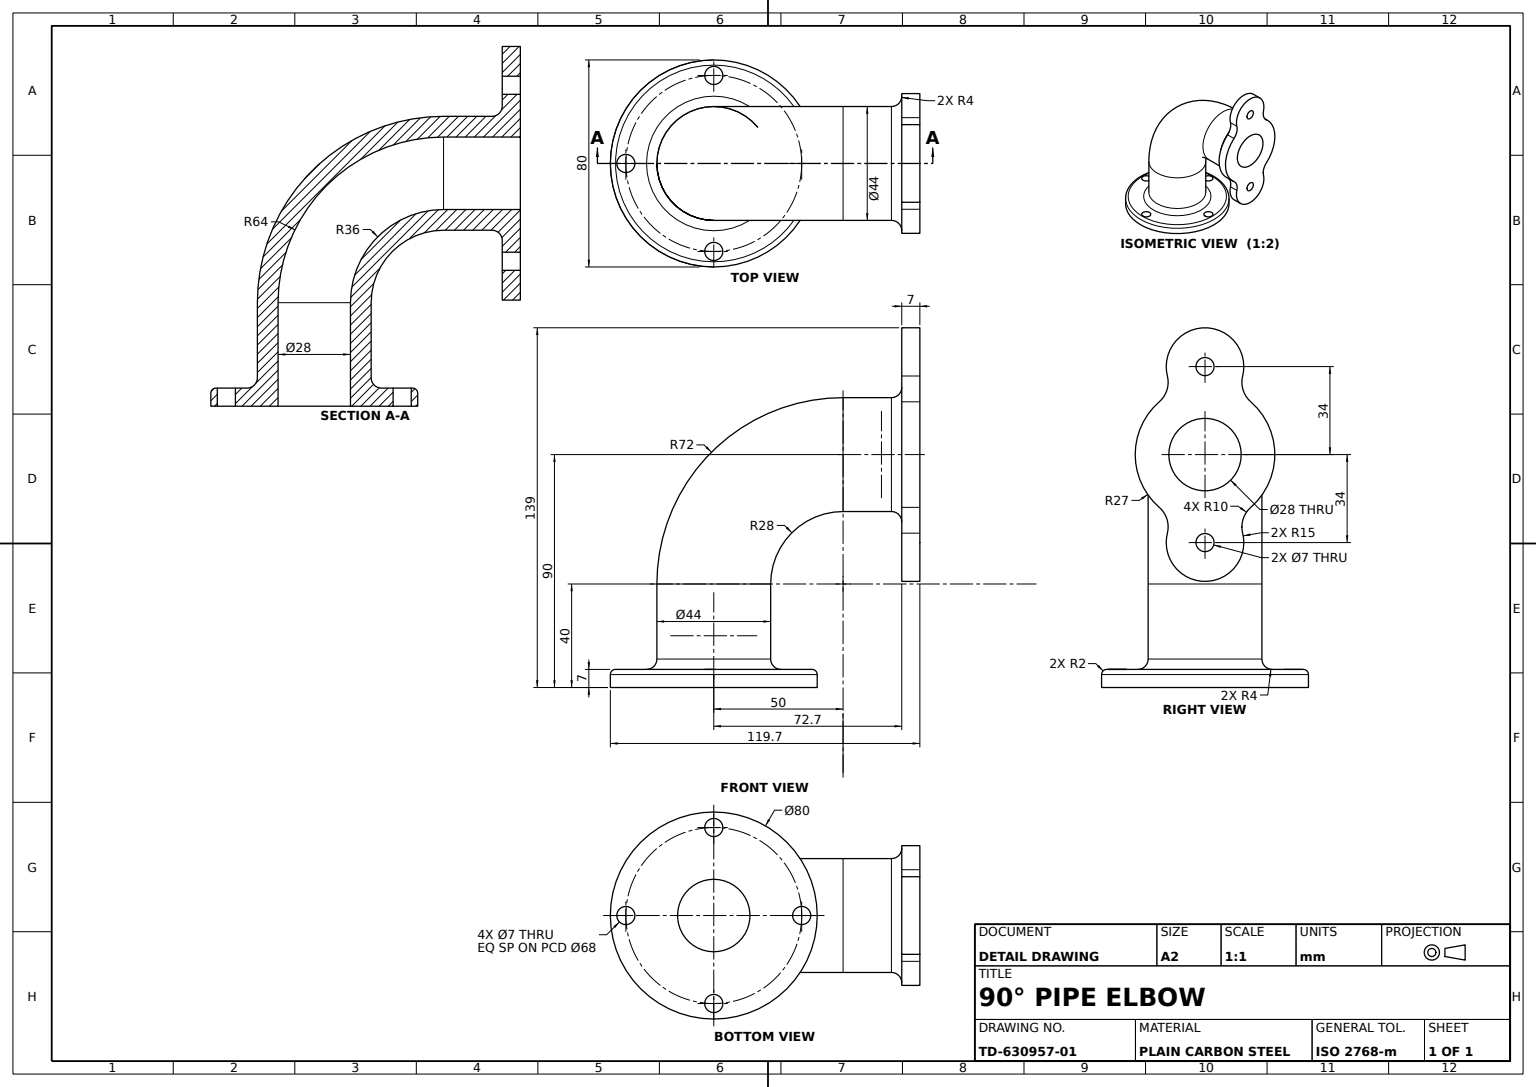
SolidWorks part; units mm, degrees
material "Plain Carbon Steel"
ref_plane "Front Plane" through (0, 0, 0) normal (0, 0, 1) x (1, 0, 0)
ref_plane "Top Plane" through (0, 0, 0) normal (0, 1, 0) x (1, 0, 0)
ref_plane "Right Plane" through (0, 0, 0) normal (1, 0, 0) x (0, 0, -1)
sketch "Oval Flange Sketch" plane through (0, 0, 0) normal (1, 0, 0) x (0, 0, -1)
  line L0 (0, -34) -> (0, 34) construction
  line L1 (0, 25) -> (0, -25) construction
  line L2 (0, -25) -> (-18.3594, -25) construction
  circle A0 centre (0, 0) radius 14
  arc A1 (17.6994, -20.3895) -> (17.6994, 20.3895) centre (0, 0) ccw
  arc A2 (14.5528, 30.3647) -> (-14.5528, 30.3647) centre (0, 34) ccw
  arc A3 (-14.5528, -30.3647) -> (14.5528, -30.3647) centre (0, -34) ccw
  circle A4 centre (0, 34) radius 3.5
  circle A5 centre (0, -34) radius 3.5
  arc A6 (-17.6994, 20.3895) -> (-17.6994, -20.3895) centre (0, 0) ccw
  arc A7 (14.5528, 30.3647) -> (17.6994, 20.3895) centre (24.2547, 27.9412) ccw
  arc A8 (-14.5528, 30.3647) -> (-17.6994, 20.3895) centre (-24.2547, 27.9412) cw
  arc A9 (17.6994, -20.3895) -> (14.5528, -30.3647) centre (24.2547, -27.9412) ccw
  arc A10 (-14.5528, -30.3647) -> (-17.6994, -20.3895) centre (-24.2547, -27.9412) ccw
  point P18 (-11.5354, 24.4118)
  dimension "D1" = 54
  dimension "D2" = 28
  dimension "D5" = 30
  dimension "D6" = 7
  dimension "D7" = 30
  dimension "D8" = 7
  dimension "D11" = 10
  dimension "D3" = 68
  dimension "D4" = 34
  dimension "D9" = 50
  dimension "D10" = 25
extrude "Oval Flange" add sketch "Oval Flange Sketch" along normal mid plane 7
sketch "Elbow Path Sketch" plane through (0, 0, 0) normal (0, 0, 1) x (1, 0, 0)
  line L0 (0, 0) -> (-26.1956, 0)
  line L1 (-76.1956, -50) -> (-76.1956, -83)
  arc A0 (-26.1956, 0) -> (-76.1956, -50) centre (-26.1956, -50) ccw
  dimension "D1" = 50
  dimension "D2" = 33
  dimension "D3" = 76.1956
ref_plane "Pipe Profile Plane" through (0, -83, 0) normal (0, 1, 0) x (1, 0, 0)
sketch "Pipe Section Sketch Ø44xØ28" plane through (0, -83, 0) normal (0, 1, 0) x (1, 0, 0)
  line L0 (-76.1956, 0) -> (-26.1956, 0) construction
  circle A0 centre (-76.1956, 0) radius 14
  circle A1 centre (-76.1956, 0) radius 22
  dimension "D1" = 28
  dimension "D2" = 44
  dimension "D3" = 76.1956
sweep "Pipe Elbow Sweep" add profiles "Pipe Section Sketch Ø44xØ28" path "Elbow Path Sketch"
sketch "Round Flange Sketch" plane through (0, -83, 0) normal (0, -1, 0) x (1, 0, 0)
  circle A0 centre (-76.1956, 0) radius 40
  circle A1 centre (-76.1956, 0) radius 14
  dimension "D1" = 80
  dimension "D2" = 28
extrude "Round Flange Ø80" add sketch "Round Flange Sketch" along normal blind 7
fillet "Pipe to Flange Fillets R4" radius 4 2 edges at (-3.5, 0, -22) (-76.1956, -83, 22)
fillet "Round Flange Edge Fillet R2" radius 2 1 edges at (-76.1956, -83, -40)
sketch "Round Flange Bolt Holes Sketch" plane through (0, -90, 0) normal (0, -1, 0) x (1, 0, 0)
  line L0 (0, 0) -> (-127.6563, 0) construction
  line L1 (-76.1956, 0) -> (-76.1956, 46.1252) construction
  line L2 (-76.1956, 0) -> (-76.1956, -48.7761) construction
  circle A0 centre (-110.1956, 0) radius 3.5
  circle A1 centre (-42.1956, 0) radius 3.5
  circle A2 centre (-76.1956, 34) radius 3.5
  circle A3 centre (-76.1956, -34) radius 3.5
  dimension "D3" = 7
  dimension "D4" = 7
  dimension "D5" = 7
  dimension "D6" = 7
  dimension "D1" = 68
  dimension "D2" = 34
  dimension "D7" = 68
  dimension "D8" = 34
extrude "Round Flange Bolt Holes 4xØ7" cut sketch "Round Flange Bolt Holes Sketch" against normal blind 10
